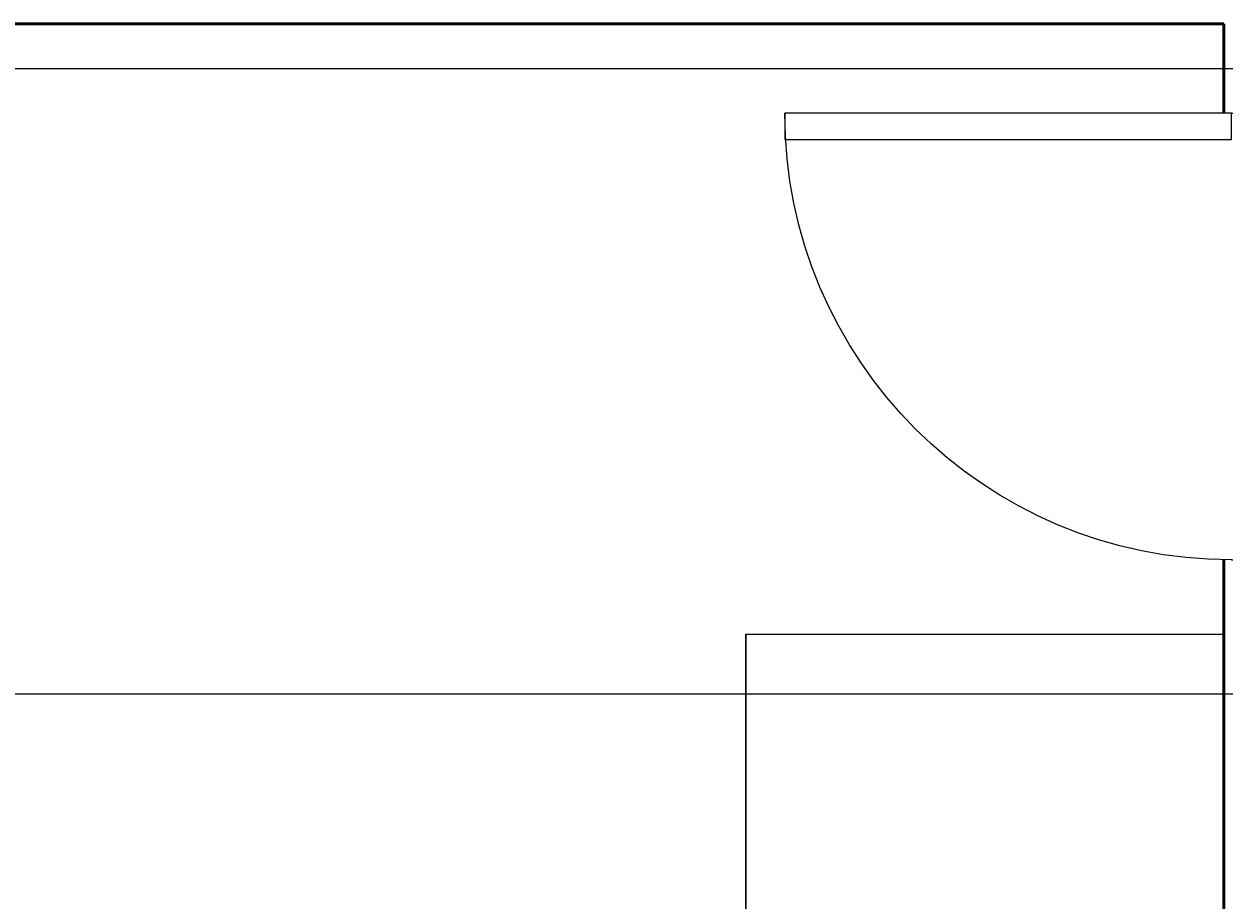
# Model space of a CAD drawing. Units: inches. Extents: x 5375 to 6084, y 16106 to 17259.
# Tile 30 of 32: x 5866 to 5946, y 16869 to 16928. Entities that reach past the tile are written whole.
import ezdxf

# ---------------------------------------------------------------- set-up
doc = ezdxf.new("R2010")
doc.units = ezdxf.units.IN
for name, color, linetype, lineweight in [('A-ANNO-DIMS', 2, 'Continuous', 18), ('A-FLOR-CASE', 3, 'Continuous', 18), ('DOOR', 4, 'Continuous', 25), ('WALL', 6, 'Continuous', 50)]:
    doc.layers.add(name, color=color, linetype=linetype, lineweight=lineweight)
doc.styles.get("Standard").update_dxf_attribs({"font": 'arial.ttf'})
doc.dimstyles.get("Standard").update_dxf_attribs({"dimtxt": 0.18, "dimasz": 0.18, "dimexe": 0.18, "dimexo": 0.0625, "dimgap": 0.09, "dimtad": 0, "dimtih": 1, "dimtoh": 1, "dimdec": 4, "dimzin": 0, "dimdsep": 46, "dimtxsty": 'Standard', "dimcen": 0.09, "dimadec": 0, "dimazin": 0, "dimtfac": 1, "dimtdec": 4, "dimtofl": 0, "dimtmove": 0, "dimatfit": 3, "dimfxl": 1, "dimtolj": 1, "dimtzin": 0, "dimarcsym": 0})

# ---------------------------------------------------------------- blocks, each defined once
blk = doc.blocks.new('*U2')
for p, q in [((0, 0), (0, -100)), ((750, 0), (750, -100))]:
    blk.add_line(p, q)
blk.add_lwpolyline([(0, 0), (0, 750), (43.75, 750), (43.75, 0)], close=True)
blk.add_arc((0, 0), 750, 0, 90)
blk = doc.blocks.new('*D41')
at = {"layer": 'A-ANNO-DIMS', "color": 0, "lineweight": -2, "transparency": 16777216}
for p, q in [((5702.182, 16924.579), (6084.2, 16924.579)), ((6084.02, 16924.399), (6084.02, 16903.76)), ((6084.02, 16882.759), (6084.02, 16903.399)), ((5702.182, 16882.579), (6084.2, 16882.579))]:
    blk.add_line(p, q, dxfattribs=at)
at = {"layer": 'A-ANNO-DIMS', "color": 0, "transparency": 16777216}
for points in [[(6083.99, 16924.399), (6084.05, 16924.399), (6084.02, 16924.579)], [(6083.99, 16882.759), (6084.05, 16882.759), (6084.02, 16882.579)]]:
    blk.add_solid(points, dxfattribs=at)
at = {"layer": 'Defpoints', "color": 0, "transparency": 16777216}
for p in [(5702.12, 16924.579), (6084.02, 16924.579), (5702.12, 16882.579)]:
    blk.add_point(p, dxfattribs=at)
at = {"layer": 'A-ANNO-DIMS', "color": 0, "transparency": 16777216, "insert": (6084.02, 16903.579), "char_height": 0.18, "attachment_point": 5}
blk.add_mtext('\\A1;42', dxfattribs=at)
blk = doc.blocks.new('*D44')
at = {"layer": 'A-ANNO-DIMS', "color": 0, "lineweight": -2, "transparency": 16777216}
for p, q in [((5914.003, 16886.533), (5914.003, 16106.483)), ((5946.12, 16886.533), (5946.12, 16106.483)), ((5914.183, 16106.663), (5929.598, 16106.663)), ((5945.94, 16106.663), (5930.525, 16106.663))]:
    blk.add_line(p, q, dxfattribs=at)
at = {"layer": 'A-ANNO-DIMS', "color": 0, "transparency": 16777216}
for points in [[(5914.183, 16106.693), (5914.183, 16106.633), (5914.003, 16106.663)], [(5945.94, 16106.693), (5945.94, 16106.633), (5946.12, 16106.663)]]:
    blk.add_solid(points, dxfattribs=at)
at = {"layer": 'Defpoints', "color": 0, "transparency": 16777216}
for p in [(5914.003, 16886.596), (5946.12, 16886.596), (5914.003, 16106.663)]:
    blk.add_point(p, dxfattribs=at)
at = {"layer": 'A-ANNO-DIMS', "color": 0, "transparency": 16777216, "insert": (5930.062, 16106.663), "char_height": 0.18, "attachment_point": 5}
blk.add_mtext('\\A1;32.117', dxfattribs=at)

msp = doc.modelspace()

# ---------------------------------------------------------------- linework, layer by layer
at = {"layer": 'A-FLOR-CASE'}
for p, q in [((5914.0033, 16809.3651), (5914.0033, 16886.5956)), ((5914.0033, 16886.5956), (5946.1199, 16886.5956))]:
    msp.add_line(p, q, dxfattribs=at)
at = {"layer": 'WALL'}
for p, q in [((5826.1199, 16927.5793), (5946.1199, 16927.5793)), ((5946.1199, 16927.5793), (5946.1199, 16921.5793)), ((5946.1199, 16891.5793), (5946.1199, 16771.5793))]:
    msp.add_line(p, q, dxfattribs=at)

# ---------------------------------------------------------------- block references
at = {"layer": 'DOOR', "xscale": -0.0399999999999999, "yscale": 0.0399999999999999, "zscale": 0.0399999999999999, "rotation": 90}
msp.add_blockref('*U2', (5946.6199, 16921.5793), dxfattribs=at)

# ---------------------------------------------------------------- dimensions: what is measured, and where the dimension line sits
at = {"layer": 'A-ANNO-DIMS'}
dim = msp.add_linear_dim(base=(6084.0199, 16924.5793), p1=(5702.1199, 16882.5793), p2=(5702.1199, 16924.5793), angle=90, dimstyle='Standard', override={"dimdec": 0, "dimlfac": 1, "dimrnd": 0, "dimzin": 0, "dimdsep": 46, "dimlunit": 2}, dxfattribs=at)
dim.commit()
dim.dimension.update_dxf_attribs({"geometry": '*D41', "text_midpoint": (6084.0199, 16903.5793)})
dim = msp.add_linear_dim(base=(5914.0033, 16106.6631), p1=(5946.1199, 16886.5956), p2=(5914.0033, 16886.5956), dimstyle='Standard', override={"dimdec": 3, "dimlfac": 1, "dimrnd": 0, "dimzin": 0, "dimdsep": 46, "dimlunit": 2}, dxfattribs=at)
dim.commit()
dim.dimension.update_dxf_attribs({"geometry": '*D44', "text_midpoint": (5930.0616, 16106.6631)})

doc.saveas('drawing.dxf')
